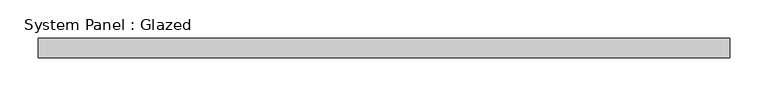
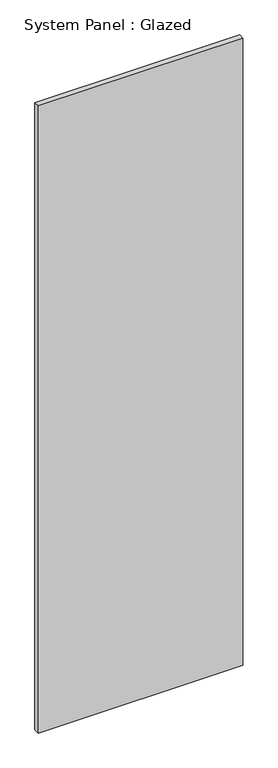
"""IFC4 building model written with IfcOpenShell, lengths in millimetres: plate geometry, System Panel : Glazed."""

from ifc_helpers import new_model, si_unit, origin, origin_with_axes, place, context, project, spatial, polyline, outline, extrude, source, transform, mapped, element, save


def system_panel_glazed_15df7e53(model_context):
    return source(origin(), model_context, "Body", "SweptSolid", [
        extrude(outline(polyline([(450.85, 19.05), (-450.85, 19.05), (-450.85, 44.45), (450.85, 44.45), (450.85, 19.05)])), origin_with_axes(), (0.0, 0.0, 1.0), 2921.0),
    ])


if __name__ == "__main__":
    model = new_model("IFC4")
    model_context = context("Model", 3, world=origin())
    ifc_project = project(units=[si_unit("LENGTHUNIT", "METRE", prefix="MILLI")], contexts=[model_context])
    site = spatial("IfcSite", under=ifc_project)
    building = spatial("IfcBuilding", under=site)
    placement = place(None, origin())
    system_panel_glazed_shape = system_panel_glazed_15df7e53(model_context)
    element("IfcPlate", 1, ObjectType="System Panel : Glazed", at=placement, inside=building, context=model_context, shape_type="MappedRepresentation", body=[
        mapped(system_panel_glazed_shape, transform((0.0, 0.0, 0.0), x_axis=(1.0, 0.0, 0.0), y_axis=(0.0, 1.0, 0.0), z_axis=(0.0, 0.0, 1.0))),
    ])
    save(model, "model.ifc")

# Revit data of these elements
# Type "System Panel : Glazed"
#   Construction Type Id = "GSP4R"
#   Analytic Construction = "1/8 in Pilkington single glazing"
#   Visual Light Transmittance = 0.9
#   Solar Heat Gain Coefficient = 0.86
#   Heat Transfer Coefficient (U) = 1.18115 BTU/(h·ft²·°F)
# Element 1 (IfcPlate, "System Panel : Glazed")
#   Materials on its faces: "Glass"
# Materials
#   "Glass": class "Glass", colour RGB 0 128 192, transparency 0.75, Description = "Soda Lime Glass", Cost = 0
